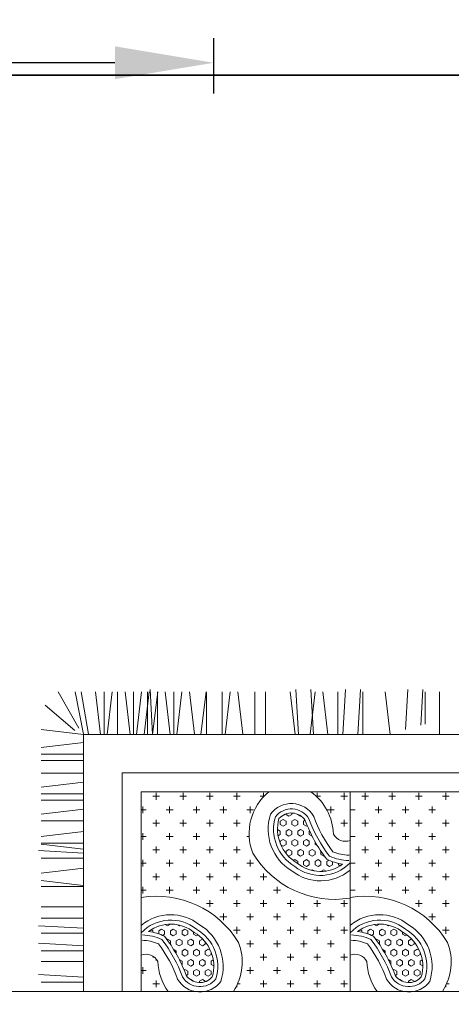
# Model space of a CAD drawing. Units: inches. Extents: x -638 to 186, y -762 to 59.
# Tile 18 of 31: x -135 to -118, y -243 to -203. Entities that reach past the tile are written whole.
import ezdxf

# ---------------------------------------------------------------- set-up
doc = ezdxf.new("R2010")
doc.units = ezdxf.units.IN
for name, color, linetype, lineweight in [('A-ANNO-DIMS', 2, 'Continuous', 18), ('furn', 8, 'Continuous', 13), ('wall', 7, 'Continuous', 35)]:
    doc.layers.add(name, color=color, linetype=linetype, lineweight=lineweight)
doc.styles.get("Standard").update_dxf_attribs({"font": 'arial.ttf'})
doc.dimstyles.new('ISO-25', dxfattribs={"dimtxt": 4, "dimasz": 4, "dimexe": 1.25, "dimexo": 0.625, "dimtad": 0, "dimlunit": 4, "dimtxsty": 'Standard', "dimcen": 2.5, "dimclrt": 256, "dimadec": 0, "dimazin": 0, "dimtfac": 1, "dimtmove": 0, "dimatfit": 3, "dimfxl": 1, "dimfxlon": 1, "dimarcsym": 0})

# ---------------------------------------------------------------- blocks, each defined once
blk = doc.blocks.new('BED-DOUBLE-WITH-NIGHTSTANDS')
for p, q in [((58.548, 11.244), (58.548, 59.951)), ((58.923, 31.914), (58.923, 33.642)), ((59.126, 31.914), (59.228, 33.743)), ((59.755, 31.928), (59.755, 33.639)), ((60.193, 31.914), (60.193, 33.642)), ((60.397, 31.914), (60.499, 33.743)), ((60.906, 31.914), (60.906, 33.642)), ((61.11, 31.914), (61.212, 33.743)), ((61.517, 31.914), (61.517, 33.642)), ((61.977, 31.914), (61.977, 33.642)), ((62.81, 31.928), (62.81, 33.639)), ((62.841, 31.928), (63.044, 33.642)), ((63.554, 31.914), (63.35, 33.642)), ((63.961, 31.914), (63.961, 33.642)), ((64.165, 31.914), (64.266, 33.743)), ((64.327, 31.928), (64.531, 33.642)), ((64.572, 31.914), (64.572, 33.642)), ((65.04, 31.914), (64.836, 33.642)), ((65.476, 31.914), (65.476, 33.642)), ((65.944, 31.914), (65.741, 33.642)), ((66.309, 31.928), (66.309, 33.639)), ((66.573, 31.914), (66.573, 33.642)), ((67.041, 31.914), (66.838, 33.642)), ((67.406, 31.928), (67.406, 33.639)), ((67.922, 31.928), (67.922, 33.639)), ((68.186, 31.914), (68.186, 33.642)), ((68.654, 31.914), (68.45, 33.642)), ((68.982, 31.914), (69.186, 33.642)), ((69.142, 32.273), (70.169, 33.468)), ((69.232, 32.112), (70.71, 32.951)), ((68.996, 31.914), (70.707, 32.257)), ((68.996, 31.721), (70.707, 32.011)), ((58.548, 31.914), (68.982, 31.914)), ((68.982, 31.914), (68.982, 1.829)), ((68.982, 31.232), (70.71, 31.436)), ((68.982, 30.966), (70.71, 30.762)), ((68.996, 31.086), (70.707, 31.086)), ((68.982, 30.547), (70.71, 30.547)), ((58.548, 30.359), (67.427, 30.359)), ((67.427, 30.359), (67.427, 3.384)), ((68.982, 30.033), (70.71, 30.237)), ((68.982, 29.767), (70.71, 29.563)), ((68.996, 29.887), (70.707, 29.887)), ((58.548, 29.582), (66.65, 29.582)), ((59.258, 29.515), (59.53, 29.515)), ((59.394, 29.379), (59.394, 29.582)), ((62.523, 29.515), (62.795, 29.515)), ((62.659, 29.379), (62.659, 29.582)), ((63.612, 29.515), (63.884, 29.515)), ((63.748, 29.379), (63.748, 29.582)), ((64.7, 29.515), (64.972, 29.515)), ((64.836, 29.379), (64.836, 29.582)), ((65.788, 29.515), (66.06, 29.515)), ((65.924, 29.379), (65.924, 29.582)), ((66.65, 29.582), (66.65, 4.161)), ((68.982, 29.46), (70.71, 29.256)), ((68.982, 29.324), (70.71, 29.324)), ((68.982, 29.121), (70.811, 29.223)), ((58.714, 28.971), (58.986, 28.971)), ((58.85, 28.835), (58.85, 29.107)), ((59.802, 28.971), (59.857, 28.971)), ((59.938, 29.054), (59.938, 29.107)), ((61.003, 28.869), (60.881, 28.869)), ((61.003, 29.104), (60.948, 29.104)), ((61.047, 29.18), (61.003, 29.104)), ((61.003, 28.869), (61.072, 28.751)), ((63.067, 28.971), (63.339, 28.971)), ((63.203, 28.835), (63.203, 29.107)), ((64.156, 28.971), (64.428, 28.971)), ((64.292, 28.835), (64.292, 29.107)), ((65.244, 28.971), (65.516, 28.971)), ((65.38, 28.835), (65.38, 29.107)), ((66.332, 28.971), (66.605, 28.971)), ((66.468, 28.835), (66.468, 29.107)), ((68.982, 28.917), (70.71, 28.917)), ((68.996, 29.116), (70.71, 28.912)), ((60.459, 28.399), (60.459, 28.397)), ((60.595, 28.397), (60.459, 28.397)), ((60.663, 28.515), (60.595, 28.397)), ((60.652, 28.534), (60.663, 28.515)), ((60.867, 28.397), (60.799, 28.28)), ((60.821, 28.713), (60.867, 28.633)), ((61.003, 28.633), (60.867, 28.633)), ((61.003, 28.397), (60.867, 28.397)), ((61.072, 28.751), (61.003, 28.633)), ((61.003, 28.397), (61.072, 28.28)), ((61.261, 28.608), (61.208, 28.515)), ((61.208, 28.515), (61.276, 28.397)), ((61.279, 28.397), (61.276, 28.397)), ((62.523, 28.427), (62.795, 28.427)), ((62.659, 28.291), (62.659, 28.563)), ((63.612, 28.427), (63.884, 28.427)), ((63.748, 28.291), (63.748, 28.563)), ((64.7, 28.427), (64.972, 28.427)), ((64.836, 28.291), (64.836, 28.563)), ((65.788, 28.427), (66.06, 28.427)), ((65.924, 28.291), (65.924, 28.563)), ((68.982, 28.403), (70.71, 28.606)), ((59.843, 28.037), (59.779, 27.926)), ((60.187, 28.162), (60.075, 28.162)), ((60.245, 28.262), (60.187, 28.162)), ((60.459, 28.162), (60.391, 28.044)), ((60.391, 28.044), (60.459, 27.926)), ((60.595, 28.162), (60.459, 28.162)), ((60.595, 28.162), (60.663, 28.044)), ((60.663, 28.044), (60.595, 27.926)), ((60.799, 28.28), (60.867, 28.162)), ((61.003, 28.162), (60.867, 28.162)), ((61.072, 28.28), (61.003, 28.162)), ((61.258, 28.131), (61.208, 28.044)), ((61.208, 28.044), (61.231, 28.004)), ((63.203, 27.747), (63.203, 28.019)), ((64.292, 27.747), (64.292, 28.019)), ((65.38, 27.747), (65.38, 28.019)), ((66.468, 27.747), (66.468, 28.019)), ((68.982, 28.136), (70.71, 27.933)), ((68.996, 28.256), (70.707, 28.256)), ((59.199, 27.753), (59.235, 27.69)), ((59.371, 27.69), (59.235, 27.69)), ((59.439, 27.808), (59.371, 27.69)), ((59.419, 27.842), (59.439, 27.808)), ((59.643, 27.69), (59.575, 27.573)), ((59.637, 27.937), (59.643, 27.926)), ((59.779, 27.926), (59.643, 27.926)), ((59.779, 27.69), (59.643, 27.69)), ((59.779, 27.69), (59.847, 27.573)), ((60.051, 27.926), (59.983, 27.808)), ((59.983, 27.808), (60.051, 27.69)), ((60.187, 27.926), (60.051, 27.926)), ((60.187, 27.69), (60.051, 27.69)), ((60.187, 27.926), (60.255, 27.808)), ((60.255, 27.808), (60.187, 27.69)), ((60.459, 27.69), (60.391, 27.573)), ((60.595, 27.926), (60.459, 27.926)), ((60.595, 27.69), (60.459, 27.69)), ((60.595, 27.69), (60.663, 27.573)), ((60.867, 27.926), (60.799, 27.808)), ((60.799, 27.808), (60.867, 27.69)), ((61.003, 27.926), (60.867, 27.926)), ((61.003, 27.69), (60.867, 27.69)), ((61.003, 27.926), (61.072, 27.808)), ((61.072, 27.808), (61.003, 27.69)), ((63.067, 27.883), (63.339, 27.883)), ((64.156, 27.883), (64.428, 27.883)), ((65.244, 27.883), (65.516, 27.883)), ((66.332, 27.883), (66.605, 27.883)), ((68.996, 27.424), (70.71, 27.627)), ((58.963, 27.219), (58.904, 27.219)), ((58.963, 27.455), (58.955, 27.455)), ((59.031, 27.573), (58.963, 27.455)), ((58.963, 27.219), (59.031, 27.101)), ((59.025, 27.583), (59.031, 27.573)), ((59.235, 27.455), (59.167, 27.337)), ((59.167, 27.337), (59.235, 27.219)), ((59.371, 27.455), (59.235, 27.455)), ((59.371, 27.219), (59.235, 27.219)), ((59.371, 27.455), (59.439, 27.337)), ((59.439, 27.337), (59.371, 27.219)), ((59.575, 27.573), (59.643, 27.455)), ((59.643, 27.219), (59.575, 27.101)), ((59.779, 27.455), (59.643, 27.455)), ((59.779, 27.219), (59.643, 27.219)), ((59.847, 27.573), (59.779, 27.455)), ((59.779, 27.219), (59.847, 27.101)), ((60.051, 27.455), (59.983, 27.337)), ((59.983, 27.337), (60.051, 27.219)), ((60.187, 27.455), (60.051, 27.455)), ((60.187, 27.219), (60.051, 27.219)), ((60.187, 27.455), (60.255, 27.337)), ((60.255, 27.337), (60.187, 27.219)), ((60.391, 27.573), (60.459, 27.455)), ((60.459, 27.219), (60.391, 27.101)), ((60.595, 27.455), (60.459, 27.455)), ((60.595, 27.219), (60.459, 27.219)), ((60.663, 27.573), (60.595, 27.455)), ((60.595, 27.219), (60.663, 27.101)), ((60.867, 27.455), (60.799, 27.337)), ((60.799, 27.337), (60.836, 27.274)), ((60.958, 27.455), (60.867, 27.455)), ((62.523, 27.339), (62.795, 27.339)), ((62.659, 27.203), (62.659, 27.475)), ((63.612, 27.339), (63.884, 27.339)), ((63.748, 27.203), (63.748, 27.475)), ((64.7, 27.339), (64.972, 27.339)), ((64.836, 27.203), (64.836, 27.475)), ((65.788, 27.339), (66.06, 27.339)), ((65.924, 27.203), (65.924, 27.475)), ((58.963, 26.984), (58.94, 26.984)), ((59.031, 27.101), (58.963, 26.984)), ((59.235, 26.984), (59.167, 26.866)), ((59.167, 26.866), (59.235, 26.748)), ((59.371, 26.984), (59.235, 26.984)), ((59.371, 26.984), (59.439, 26.866)), ((59.439, 26.866), (59.371, 26.748)), ((59.575, 27.101), (59.643, 26.984)), ((59.779, 26.984), (59.643, 26.984)), ((59.847, 27.101), (59.779, 26.984)), ((60.051, 26.984), (59.983, 26.866)), ((59.983, 26.866), (60.051, 26.748)), ((60.187, 26.984), (60.051, 26.984)), ((60.187, 26.984), (60.255, 26.866)), ((60.255, 26.866), (60.201, 26.772)), ((60.391, 27.101), (60.459, 26.984)), ((60.553, 26.984), (60.459, 26.984)), ((60.663, 27.101), (60.637, 27.055)), ((61.979, 26.795), (62.251, 26.795)), ((62.115, 26.659), (62.115, 26.931)), ((63.067, 26.795), (63.339, 26.795)), ((63.203, 26.659), (63.203, 26.931)), ((64.156, 26.795), (64.428, 26.795)), ((64.292, 26.659), (64.292, 26.931)), ((65.244, 26.795), (65.516, 26.795)), ((65.38, 26.659), (65.38, 26.931)), ((66.332, 26.795), (66.605, 26.795)), ((66.468, 26.659), (66.468, 26.931)), ((68.996, 27.156), (70.71, 26.953)), ((68.996, 26.933), (70.707, 26.933)), ((59.371, 26.748), (59.235, 26.748)), ((59.643, 26.748), (59.58, 26.638)), ((59.779, 26.748), (59.643, 26.748)), ((59.779, 26.748), (59.83, 26.661)), ((60.144, 26.748), (60.051, 26.748)), ((61.435, 26.25), (61.707, 26.25)), ((61.571, 26.114), (61.571, 26.386)), ((62.523, 26.25), (62.795, 26.25)), ((62.659, 26.114), (62.659, 26.386)), ((63.612, 26.25), (63.884, 26.25)), ((63.748, 26.114), (63.748, 26.386)), ((64.7, 26.25), (64.972, 26.25)), ((64.836, 26.114), (64.836, 26.386)), ((65.788, 26.25), (66.06, 26.25)), ((65.924, 26.114), (65.924, 26.386)), ((68.982, 26.177), (70.71, 25.974)), ((68.996, 26.297), (70.707, 26.297)), ((58.714, 25.706), (58.783, 25.706)), ((58.85, 25.57), (58.85, 25.675)), ((60.891, 25.706), (61.163, 25.706)), ((61.027, 25.57), (61.027, 25.842)), ((61.979, 25.706), (62.251, 25.706)), ((62.115, 25.57), (62.115, 25.842)), ((63.067, 25.706), (63.339, 25.706)), ((63.203, 25.57), (63.203, 25.842)), ((64.156, 25.706), (64.428, 25.706)), ((64.292, 25.57), (64.292, 25.842)), ((65.244, 25.706), (65.516, 25.706)), ((65.38, 25.57), (65.38, 25.842)), ((66.332, 25.706), (66.605, 25.706)), ((66.468, 25.57), (66.468, 25.842)), ((68.996, 25.465), (70.71, 25.668)), ((59.394, 25.026), (59.394, 25.298)), ((60.483, 25.026), (60.483, 25.298)), ((61.571, 25.026), (61.571, 25.298)), ((62.659, 25.026), (62.659, 25.298)), ((63.748, 25.026), (63.748, 25.298)), ((64.836, 25.2), (64.836, 25.298)), ((65.924, 25.026), (65.924, 25.298)), ((59.258, 25.162), (59.53, 25.162)), ((60.346, 25.162), (60.619, 25.162)), ((61.435, 25.162), (61.707, 25.162)), ((62.523, 25.162), (62.795, 25.162)), ((63.612, 25.162), (63.884, 25.162)), ((65.788, 25.162), (66.06, 25.162)), ((68.996, 24.973), (70.707, 24.973)), ((58.714, 24.618), (58.986, 24.618)), ((58.85, 24.482), (58.85, 24.754)), ((59.802, 24.618), (60.074, 24.618)), ((59.938, 24.482), (59.938, 24.754)), ((60.891, 24.618), (61.163, 24.618)), ((61.027, 24.482), (61.027, 24.754)), ((61.979, 24.618), (62.251, 24.618)), ((62.115, 24.482), (62.115, 24.754)), ((63.067, 24.618), (63.339, 24.618)), ((63.203, 24.482), (63.203, 24.754)), ((66.45, 24.618), (66.605, 24.618)), ((66.468, 24.601), (66.468, 24.754)), ((68.996, 24.543), (70.707, 24.543)), ((59.258, 24.074), (59.53, 24.074)), ((59.394, 23.938), (59.394, 24.21)), ((60.346, 24.074), (60.619, 24.074)), ((60.483, 23.938), (60.483, 24.21)), ((61.435, 24.074), (61.707, 24.074)), ((61.571, 23.938), (61.571, 24.21)), ((62.523, 24.074), (62.795, 24.074)), ((62.659, 23.938), (62.659, 24.21)), ((64.917, 23.942), (64.866, 24.03)), ((65.053, 23.942), (65.116, 24.052)), ((58.85, 23.393), (58.85, 23.666)), ((59.938, 23.393), (59.938, 23.666)), ((61.027, 23.393), (61.027, 23.666)), ((62.115, 23.393), (62.115, 23.666)), ((64.032, 23.589), (64.059, 23.635)), ((64.143, 23.707), (64.236, 23.707)), ((64.304, 23.589), (64.236, 23.707)), ((64.44, 23.825), (64.495, 23.919)), ((64.508, 23.707), (64.44, 23.825)), ((64.508, 23.707), (64.644, 23.707)), ((64.552, 23.942), (64.644, 23.942)), ((64.712, 23.825), (64.644, 23.942)), ((64.644, 23.707), (64.712, 23.825)), ((64.849, 23.589), (64.917, 23.707)), ((64.917, 23.942), (65.053, 23.942)), ((64.917, 23.707), (65.053, 23.707)), ((65.121, 23.589), (65.053, 23.707)), ((65.257, 23.825), (65.325, 23.942)), ((65.325, 23.707), (65.257, 23.825)), ((65.325, 23.942), (65.461, 23.942)), ((65.325, 23.707), (65.461, 23.707)), ((65.529, 23.825), (65.461, 23.942)), ((65.461, 23.707), (65.529, 23.825)), ((65.665, 23.589), (65.733, 23.707)), ((65.733, 23.707), (65.755, 23.707)), ((58.714, 23.53), (58.986, 23.53)), ((59.802, 23.53), (60.074, 23.53)), ((60.891, 23.53), (61.163, 23.53)), ((61.979, 23.53), (62.251, 23.53)), ((63.737, 23.235), (63.828, 23.235)), ((63.828, 23.235), (63.896, 23.353)), ((63.896, 23.353), (63.86, 23.416)), ((64.1, 23.471), (64.032, 23.589)), ((64.032, 23.118), (64.1, 23.235)), ((64.1, 23.471), (64.236, 23.471)), ((64.1, 23.235), (64.236, 23.235)), ((64.236, 23.471), (64.304, 23.589)), ((64.304, 23.118), (64.236, 23.235)), ((64.44, 23.353), (64.508, 23.471)), ((64.508, 23.235), (64.44, 23.353)), ((64.508, 23.471), (64.644, 23.471)), ((64.508, 23.235), (64.644, 23.235)), ((64.712, 23.353), (64.644, 23.471)), ((64.644, 23.235), (64.712, 23.353)), ((64.917, 23.471), (64.849, 23.589)), ((64.849, 23.118), (64.917, 23.235)), ((64.917, 23.471), (65.053, 23.471)), ((64.917, 23.235), (65.053, 23.235)), ((65.053, 23.471), (65.121, 23.589)), ((65.121, 23.118), (65.053, 23.235)), ((65.257, 23.353), (65.325, 23.471)), ((65.325, 23.235), (65.257, 23.353)), ((65.325, 23.471), (65.461, 23.471)), ((65.325, 23.235), (65.461, 23.235)), ((65.529, 23.353), (65.461, 23.471)), ((65.461, 23.235), (65.529, 23.353)), ((65.733, 23.471), (65.665, 23.589)), ((65.665, 23.118), (65.733, 23.235)), ((65.733, 23.471), (65.791, 23.471)), ((65.733, 23.235), (65.741, 23.235)), ((68.982, 23.339), (70.71, 23.542)), ((68.982, 23.207), (70.811, 23.309)), ((59.258, 22.985), (59.53, 22.985)), ((59.394, 22.849), (59.394, 23.121)), ((60.346, 22.985), (60.619, 22.985)), ((60.483, 22.849), (60.483, 23.121)), ((61.435, 22.985), (61.707, 22.985)), ((61.571, 22.849), (61.571, 23.121)), ((63.624, 22.882), (63.692, 23)), ((63.692, 22.764), (63.624, 22.882)), ((63.692, 23), (63.828, 23)), ((63.896, 22.882), (63.828, 23)), ((63.828, 22.764), (63.896, 22.882)), ((64.1, 23), (64.032, 23.118)), ((64.1, 23), (64.236, 23)), ((64.236, 23), (64.304, 23.118)), ((64.44, 22.882), (64.508, 23)), ((64.508, 22.764), (64.44, 22.882)), ((64.508, 23), (64.644, 23)), ((64.712, 22.882), (64.644, 23)), ((64.644, 22.764), (64.712, 22.882)), ((64.917, 23), (64.849, 23.118)), ((64.917, 23), (65.053, 23)), ((65.053, 23), (65.121, 23.118)), ((65.257, 22.882), (65.325, 23)), ((65.276, 22.848), (65.257, 22.882)), ((65.325, 23), (65.461, 23)), ((65.497, 22.937), (65.461, 23)), ((65.671, 23.107), (65.665, 23.118)), ((58.714, 22.441), (58.986, 22.441)), ((58.85, 22.305), (58.85, 22.577)), ((59.802, 22.441), (60.074, 22.441)), ((59.938, 22.305), (59.938, 22.577)), ((60.891, 22.441), (61.163, 22.441)), ((61.027, 22.305), (61.027, 22.577)), ((61.979, 22.441), (62.251, 22.441)), ((62.115, 22.305), (62.115, 22.577)), ((63.438, 22.559), (63.488, 22.646)), ((63.488, 22.646), (63.465, 22.686)), ((63.624, 22.411), (63.692, 22.529)), ((63.692, 22.293), (63.624, 22.411)), ((63.692, 22.764), (63.828, 22.764)), ((63.692, 22.529), (63.828, 22.529)), ((63.896, 22.411), (63.828, 22.529)), ((63.828, 22.293), (63.896, 22.411)), ((64.032, 22.646), (64.1, 22.764)), ((64.1, 22.529), (64.032, 22.646)), ((64.1, 22.764), (64.236, 22.764)), ((64.1, 22.529), (64.236, 22.529)), ((64.304, 22.646), (64.236, 22.764)), ((64.236, 22.529), (64.304, 22.646)), ((64.451, 22.428), (64.508, 22.529)), ((64.508, 22.764), (64.644, 22.764)), ((64.508, 22.529), (64.621, 22.529)), ((64.852, 22.653), (64.917, 22.764)), ((64.917, 22.764), (65.053, 22.764)), ((65.059, 22.753), (65.053, 22.764)), ((66.43, 22.441), (66.605, 22.441)), ((66.468, 22.305), (66.468, 22.481)), ((68.982, 22.596), (70.811, 22.698)), ((68.996, 22.728), (70.71, 22.524)), ((59.394, 21.761), (59.394, 22.033)), ((60.483, 21.761), (60.483, 22.033)), ((61.571, 21.761), (61.571, 22.033)), ((63.417, 22.293), (63.42, 22.293)), ((63.488, 22.175), (63.42, 22.293)), ((63.434, 22.082), (63.488, 22.175)), ((63.624, 21.939), (63.692, 22.057)), ((63.692, 22.293), (63.828, 22.293)), ((63.692, 22.057), (63.828, 22.057)), ((63.874, 21.977), (63.828, 22.057)), ((64.032, 22.175), (64.1, 22.293)), ((64.043, 22.156), (64.032, 22.175)), ((64.1, 22.293), (64.236, 22.293)), ((64.237, 22.292), (64.236, 22.293)), ((65.924, 21.761), (65.924, 22.033)), ((68.982, 22.015), (70.71, 22.219)), ((59.258, 21.897), (59.53, 21.897)), ((60.346, 21.897), (60.619, 21.897)), ((61.435, 21.897), (61.707, 21.897)), ((63.692, 21.822), (63.624, 21.939)), ((63.692, 21.822), (63.815, 21.822)), ((65.788, 21.897), (66.06, 21.897)), ((68.982, 21.608), (70.71, 21.608)), ((58.714, 21.353), (58.986, 21.353)), ((58.85, 21.217), (58.85, 21.489)), ((59.802, 21.353), (60.074, 21.353)), ((59.938, 21.217), (59.938, 21.489)), ((60.891, 21.353), (61.163, 21.353)), ((61.027, 21.217), (61.027, 21.489)), ((61.979, 21.353), (62.251, 21.353)), ((62.115, 21.217), (62.115, 21.489)), ((63.648, 21.51), (63.692, 21.586)), ((63.692, 21.586), (63.748, 21.586)), ((65.244, 21.353), (65.516, 21.353)), ((65.38, 21.217), (65.38, 21.489)), ((66.332, 21.353), (66.605, 21.353)), ((66.468, 21.217), (66.468, 21.489)), ((68.982, 21.404), (70.811, 21.302)), ((58.548, 21.108), (66.65, 21.108)), ((62.659, 20.906), (62.659, 21.108)), ((63.748, 20.906), (63.748, 21.108)), ((64.836, 20.906), (64.836, 21.108)), ((65.924, 20.906), (65.924, 21.108)), ((68.982, 20.793), (70.811, 20.691)), ((61.003, 20.395), (60.881, 20.395)), ((61.003, 20.631), (60.948, 20.631)), ((61.047, 20.707), (61.003, 20.631)), ((61.003, 20.395), (61.072, 20.277)), ((63.067, 20.498), (63.339, 20.498)), ((63.203, 20.362), (63.203, 20.634)), ((64.156, 20.498), (64.428, 20.498)), ((64.292, 20.362), (64.292, 20.634)), ((65.244, 20.498), (65.516, 20.498)), ((65.38, 20.362), (65.38, 20.634)), ((66.332, 20.498), (66.605, 20.498)), ((66.468, 20.362), (66.468, 20.634)), ((68.982, 20.59), (70.71, 20.59)), ((60.663, 20.042), (60.595, 19.924)), ((60.652, 20.061), (60.663, 20.042)), ((60.821, 20.239), (60.867, 20.159)), ((61.003, 20.159), (60.867, 20.159)), ((61.072, 20.277), (61.003, 20.159)), ((61.261, 20.135), (61.208, 20.042)), ((61.208, 20.042), (61.276, 19.924)), ((62.659, 19.817), (62.659, 20.09)), ((63.748, 19.817), (63.748, 20.09)), ((64.836, 19.817), (64.836, 20.09)), ((65.924, 19.817), (65.924, 20.09)), ((60.187, 19.688), (60.075, 19.688)), ((60.245, 19.788), (60.187, 19.688)), ((60.459, 19.688), (60.391, 19.57)), ((60.459, 19.925), (60.459, 19.924)), ((60.595, 19.924), (60.459, 19.924)), ((60.595, 19.688), (60.459, 19.688)), ((60.595, 19.688), (60.663, 19.57)), ((60.867, 19.924), (60.799, 19.806)), ((60.799, 19.806), (60.867, 19.688)), ((61.003, 19.924), (60.867, 19.924)), ((61.003, 19.688), (60.867, 19.688)), ((61.003, 19.924), (61.072, 19.806)), ((61.072, 19.806), (61.003, 19.688)), ((61.258, 19.657), (61.208, 19.57)), ((61.279, 19.924), (61.276, 19.924)), ((62.523, 19.954), (62.795, 19.954)), ((63.612, 19.954), (63.884, 19.954)), ((64.7, 19.954), (64.972, 19.954)), ((65.788, 19.954), (66.06, 19.954)), ((68.982, 19.485), (70.71, 19.689)), ((59.199, 19.28), (59.235, 19.217)), ((59.371, 19.217), (59.235, 19.217)), ((59.439, 19.335), (59.371, 19.217)), ((59.419, 19.369), (59.439, 19.335)), ((59.643, 19.217), (59.575, 19.099)), ((59.637, 19.464), (59.643, 19.453)), ((59.779, 19.453), (59.643, 19.453)), ((59.779, 19.217), (59.643, 19.217)), ((59.843, 19.564), (59.779, 19.453)), ((59.779, 19.217), (59.847, 19.099)), ((60.051, 19.453), (59.983, 19.335)), ((59.983, 19.335), (60.051, 19.217)), ((60.187, 19.453), (60.051, 19.453)), ((60.187, 19.217), (60.051, 19.217)), ((60.187, 19.453), (60.255, 19.335)), ((60.255, 19.335), (60.187, 19.217)), ((60.391, 19.57), (60.459, 19.453)), ((60.459, 19.217), (60.391, 19.099)), ((60.595, 19.453), (60.459, 19.453)), ((60.595, 19.217), (60.459, 19.217)), ((60.663, 19.57), (60.595, 19.453)), ((60.595, 19.217), (60.663, 19.099)), ((60.867, 19.453), (60.799, 19.335)), ((60.799, 19.335), (60.867, 19.217)), ((61.003, 19.453), (60.867, 19.453)), ((61.003, 19.217), (60.867, 19.217)), ((61.003, 19.453), (61.072, 19.335)), ((61.072, 19.335), (61.003, 19.217)), ((61.208, 19.57), (61.231, 19.53)), ((63.067, 19.409), (63.339, 19.409)), ((63.203, 19.273), (63.203, 19.545)), ((64.156, 19.409), (64.428, 19.409)), ((64.292, 19.273), (64.292, 19.545)), ((65.244, 19.409), (65.516, 19.409)), ((65.38, 19.273), (65.38, 19.545)), ((66.332, 19.409), (66.605, 19.409)), ((66.468, 19.273), (66.468, 19.545)), ((58.963, 18.981), (58.955, 18.981)), ((59.031, 19.099), (58.963, 18.981)), ((59.025, 19.109), (59.031, 19.099)), ((59.235, 18.981), (59.167, 18.863)), ((59.167, 18.863), (59.235, 18.746)), ((59.371, 18.981), (59.235, 18.981)), ((59.371, 18.981), (59.439, 18.863)), ((59.439, 18.863), (59.371, 18.746)), ((59.575, 19.099), (59.643, 18.981)), ((59.779, 18.981), (59.643, 18.981)), ((59.847, 19.099), (59.779, 18.981)), ((60.051, 18.981), (59.983, 18.863)), ((59.983, 18.863), (60.051, 18.746)), ((60.187, 18.981), (60.051, 18.981)), ((60.187, 18.981), (60.255, 18.863)), ((60.255, 18.863), (60.187, 18.746)), ((60.391, 19.099), (60.459, 18.981)), ((60.595, 18.981), (60.459, 18.981)), ((60.663, 19.099), (60.595, 18.981)), ((60.867, 18.981), (60.799, 18.863)), ((60.799, 18.863), (60.836, 18.801)), ((60.958, 18.981), (60.867, 18.981)), ((62.523, 18.865), (62.795, 18.865)), ((62.659, 18.729), (62.659, 19.001)), ((63.612, 18.865), (63.884, 18.865)), ((63.748, 18.729), (63.748, 19.001)), ((64.7, 18.865), (64.972, 18.865)), ((64.836, 18.729), (64.836, 19.001)), ((65.788, 18.865), (66.06, 18.865)), ((65.924, 18.729), (65.924, 19.001)), ((69.184, 18.863), (70.811, 18.772)), ((58.963, 18.746), (58.904, 18.746)), ((58.963, 18.51), (58.94, 18.51)), ((58.963, 18.746), (59.031, 18.628)), ((59.031, 18.628), (58.963, 18.51)), ((59.235, 18.51), (59.167, 18.392)), ((59.167, 18.392), (59.235, 18.274)), ((59.371, 18.746), (59.235, 18.746)), ((59.371, 18.51), (59.235, 18.51)), ((59.371, 18.51), (59.439, 18.392)), ((59.439, 18.392), (59.371, 18.274)), ((59.643, 18.746), (59.575, 18.628)), ((59.575, 18.628), (59.643, 18.51)), ((59.779, 18.746), (59.643, 18.746)), ((59.779, 18.51), (59.643, 18.51)), ((59.779, 18.746), (59.847, 18.628)), ((59.847, 18.628), (59.779, 18.51)), ((60.051, 18.51), (59.983, 18.392)), ((59.983, 18.392), (60.051, 18.274)), ((60.187, 18.746), (60.051, 18.746)), ((60.187, 18.51), (60.051, 18.51)), ((60.187, 18.51), (60.255, 18.392)), ((60.255, 18.392), (60.201, 18.298)), ((60.459, 18.746), (60.391, 18.628)), ((60.391, 18.628), (60.459, 18.51)), ((60.595, 18.746), (60.459, 18.746)), ((60.553, 18.51), (60.459, 18.51)), ((60.595, 18.746), (60.663, 18.628)), ((60.663, 18.628), (60.637, 18.582)), ((62.115, 18.185), (62.115, 18.457)), ((63.203, 18.185), (63.203, 18.457)), ((64.292, 18.185), (64.292, 18.457)), ((65.38, 18.185), (65.38, 18.457)), ((66.468, 18.185), (66.468, 18.457)), ((59.371, 18.274), (59.235, 18.274)), ((59.643, 18.274), (59.58, 18.165)), ((59.779, 18.274), (59.643, 18.274)), ((59.779, 18.274), (59.83, 18.187)), ((60.144, 18.274), (60.051, 18.274)), ((61.979, 18.321), (62.251, 18.321)), ((63.067, 18.321), (63.339, 18.321)), ((64.156, 18.321), (64.428, 18.321)), ((65.244, 18.321), (65.516, 18.321)), ((66.332, 18.321), (66.605, 18.321)), ((69.357, 18.243), (70.811, 18.162)), ((69.393, 18.06), (70.71, 18.06)), ((61.435, 17.777), (61.707, 17.777)), ((61.571, 17.641), (61.571, 17.913)), ((62.523, 17.777), (62.795, 17.777)), ((62.659, 17.641), (62.659, 17.913)), ((63.612, 17.777), (63.884, 17.777)), ((63.748, 17.641), (63.748, 17.913)), ((64.7, 17.777), (64.972, 17.777)), ((64.836, 17.641), (64.836, 17.913)), ((65.788, 17.777), (66.06, 17.777)), ((65.924, 17.641), (65.924, 17.913)), ((58.714, 17.233), (58.783, 17.233)), ((58.85, 17.097), (58.85, 17.202)), ((60.891, 17.233), (61.163, 17.233)), ((61.027, 17.097), (61.027, 17.369)), ((61.979, 17.233), (62.251, 17.233)), ((62.115, 17.097), (62.115, 17.369)), ((63.067, 17.233), (63.339, 17.233)), ((63.203, 17.097), (63.203, 17.369)), ((64.156, 17.233), (64.428, 17.233)), ((64.292, 17.097), (64.292, 17.369)), ((65.244, 17.233), (65.516, 17.233)), ((65.38, 17.097), (65.38, 17.369)), ((66.332, 17.233), (66.605, 17.233)), ((66.468, 17.097), (66.468, 17.369)), ((68.982, 17.492), (70.707, 17.492))]:
    blk.add_line(p, q)
for centre, radius, start, end in [((59.514, 29.388), 0.54, 297.0088, 21.0409), ((58.736, 29.604), 1.887, 337.4091, 358.0373), ((58.53, 28.957), 3.88, 301.1125, 9.2666), ((58.736, 29.604), 2.104, 335.7609, 358.0373), ((58.736, 29.604), 2.268, 334.7059, 351.7535), ((59.782, 28.381), 1.66, 321.1107, 46.3387), ((59.782, 28.381), 1.497, 320.6541, 36.833), ((59.782, 28.381), 1.878, 321.5973, 39.7611), ((59.856, 26.664), 2.246, 92.4675, 125.6302), ((57.143, 33.342), 5.571, 289.9219, 306.7677), ((57.143, 33.342), 5.789, 290.1318, 307.346), ((57.143, 33.342), 5.952, 290.2997, 307.7385), ((59.57, 27.2), 1.047, 120.344, 234.0192), ((59.57, 27.2), 0.829, 121.6232, 231.6957), ((59.57, 27.2), 0.666, 122.9498, 229.099), ((59.563, 28.229), 1.972, 252.055, 329.019), ((59.563, 28.229), 1.754, 253.2189, 329.4808), ((59.563, 28.229), 1.591, 254.3738, 329.9117), ((59.74, 27.689), 2.202, 237.1993, 291.1583), ((64.955, 23.002), 2.202, 39.6653, 111.1583), ((66.165, 21.733), 3.88, 121.1125, 189.2666), ((65.133, 22.461), 1.972, 72.055, 149.019), ((65.133, 22.461), 1.754, 73.2189, 149.4808), ((65.133, 22.461), 1.591, 74.3738, 149.9117), ((65.126, 23.49), 0.666, 302.9498, 49.099), ((65.126, 23.49), 0.829, 301.6232, 51.6957), ((65.126, 23.49), 1.047, 300.344, 54.0192), ((64.914, 22.31), 1.878, 141.5973, 219.7611), ((64.914, 22.31), 1.66, 141.1107, 226.3387), ((64.914, 22.31), 1.497, 140.6541, 216.833), ((67.553, 17.348), 5.952, 110.2997, 127.7385), ((67.553, 17.348), 5.789, 110.1318, 127.346), ((67.553, 17.348), 5.571, 109.9219, 126.7677), ((64.84, 24.027), 2.246, 272.4675, 323.7193), ((65.96, 21.087), 2.268, 154.7059, 171.7535), ((65.96, 21.087), 2.104, 155.7609, 178.0373), ((65.96, 21.087), 1.887, 157.4091, 178.0373), ((65.181, 21.302), 0.54, 117.0088, 201.0409), ((59.514, 20.915), 0.54, 297.0088, 21.0409), ((58.736, 21.13), 1.887, 337.4091, 358.0373), ((58.53, 20.484), 3.88, 301.1125, 9.2666), ((58.736, 21.13), 2.104, 335.7609, 358.0373), ((58.736, 21.13), 2.268, 334.7059, 351.7535), ((59.782, 19.907), 1.66, 321.1107, 46.3387), ((59.782, 19.907), 1.497, 320.6541, 36.833), ((59.782, 19.907), 1.878, 321.5973, 39.7611), ((59.856, 18.19), 2.246, 92.4675, 125.6302), ((57.143, 24.868), 5.571, 289.9219, 306.7677), ((57.143, 24.868), 5.789, 290.1318, 307.346), ((57.143, 24.868), 5.952, 290.2997, 307.7385), ((59.57, 18.727), 1.047, 120.344, 234.0192), ((59.57, 18.727), 0.829, 121.6232, 231.6957), ((59.57, 18.727), 0.666, 122.9498, 229.099), ((59.563, 19.756), 1.754, 253.2189, 329.4808), ((59.563, 19.756), 1.591, 254.3738, 329.9117), ((59.563, 19.756), 1.972, 252.055, 329.019), ((59.74, 19.215), 2.202, 237.1993, 291.1583)]:
    blk.add_arc(centre, radius, start, end)
blk = doc.blocks.new('*D23')
at = {"layer": 'A-ANNO-DIMS', "color": 0, "lineweight": -2, "transparency": 16777216}
for p, q in [((-165.015, -204.032), (-165.015, -206.282)), ((-127.219, -204.032), (-127.219, -206.282)), ((-165.015, -205.032), (-169.015, -205.032)), ((-131.219, -205.032), (-161.015, -205.032))]:
    blk.add_line(p, q, dxfattribs=at)
at = {"layer": 'A-ANNO-DIMS', "color": 0, "lineweight": 30, "transparency": 16777216}
for points in [[(-161.015, -204.365), (-161.015, -205.699), (-165.015, -205.032)], [(-131.219, -204.365), (-131.219, -205.699), (-127.219, -205.032)]]:
    blk.add_solid(points, dxfattribs=at)
at = {"layer": 'Defpoints', "color": 0, "lineweight": 30, "transparency": 16777216}
for p in [(-165.015, -199.363), (-127.219, -199.363), (-165.015, -205.032)]:
    blk.add_point(p, dxfattribs=at)
at = {"layer": 'A-ANNO-DIMS', "transparency": 16777216, "insert": (-201.224, -205.032), "char_height": 4, "attachment_point": 5}
blk.add_mtext('SWING DOOR 3\'-2" TYP.', dxfattribs=at)
blk = doc.blocks.new('*D37')
at = {"layer": 'A-ANNO-DIMS', "color": 0, "lineweight": -2, "transparency": 16777216}
for p, q in [((182.663, -232.533), (184.913, -232.533)), ((183.663, -236.533), (183.663, -250.511)), ((183.663, -276.533), (183.663, -262.555)), ((182.663, -280.533), (184.913, -280.533))]:
    blk.add_line(p, q, dxfattribs=at)
at = {"layer": 'A-ANNO-DIMS', "color": 0, "lineweight": 30, "transparency": 16777216}
for points in [[(182.997, -236.533), (184.33, -236.533), (183.663, -232.533)], [(182.997, -276.533), (184.33, -276.533), (183.663, -280.533)]]:
    blk.add_solid(points, dxfattribs=at)
at = {"layer": 'Defpoints', "color": 0, "lineweight": 30, "transparency": 16777216}
for p in [(-404.526, -232.533), (-404.526, -280.533), (183.663, -280.533)]:
    blk.add_point(p, dxfattribs=at)
at = {"layer": 'A-ANNO-DIMS', "transparency": 16777216, "insert": (183.663, -256.533), "char_height": 4, "attachment_point": 5, "rotation": 90}
blk.add_mtext('4\'-0"', dxfattribs=at)
blk = doc.blocks.new('*D56')
at = {"layer": 'A-ANNO-DIMS', "color": 0, "lineweight": -2, "transparency": 16777216}
for p, q in [((-165.026, 52.017), (-165.026, 54.267)), ((-100.526, 52.017), (-100.526, 54.267)), ((-161.026, 53.017), (-143.378, 53.017)), ((-104.526, 53.017), (-122.174, 53.017))]:
    blk.add_line(p, q, dxfattribs=at)
at = {"layer": 'A-ANNO-DIMS', "color": 0, "lineweight": 30, "transparency": 16777216}
for points in [[(-161.026, 53.684), (-161.026, 52.35), (-165.026, 53.017)], [(-104.526, 53.684), (-104.526, 52.35), (-100.526, 53.017)]]:
    blk.add_solid(points, dxfattribs=at)
at = {"layer": 'Defpoints', "color": 0, "lineweight": 30, "transparency": 16777216}
for p in [(-100.526, 53.017), (-165.026, -408.033), (-100.526, -408.033)]:
    blk.add_point(p, dxfattribs=at)
at = {"layer": 'A-ANNO-DIMS', "transparency": 16777216, "insert": (-132.776, 53.017), "char_height": 4, "attachment_point": 5}
blk.add_mtext('5\'-4 1/2"', dxfattribs=at)

msp = doc.modelspace()

# ---------------------------------------------------------------- linework, layer by layer
at = {"layer": 'wall'}
msp.add_line((-160.526, -205.533), (1.474, -205.533), dxfattribs=at)

# ---------------------------------------------------------------- block references
at = {"layer": 'furn', "rotation": 90.00000000000006}
msp.add_blockref('BED-DOUBLE-WITH-NIGHTSTANDS', (-100.575, -301.287), dxfattribs=at)

# ---------------------------------------------------------------- dimensions: what is measured, and where the dimension line sits
at = {"layer": 'A-ANNO-DIMS'}
dim = msp.add_linear_dim(base=(-100.526, 53.017), p1=(-165.026, -408.033), p2=(-100.526, -408.033), dimstyle='ISO-25', override={"dimdec": 1, "dimlfac": 1, "dimrnd": 0, "dimzin": 1, "dimdsep": 46, "dimlunit": 4, "dimfrac": 2}, dxfattribs=at)
dim.commit()
dim.dimension.update_dxf_attribs({"geometry": '*D56', "text_midpoint": (-132.776, 53.017)})
dim = msp.add_linear_dim(base=(-165.015, -205.032), p1=(-127.219, -199.363), p2=(-165.015, -199.363), angle=180, text='SWING DOOR <> TYP.', dimstyle='ISO-25', override={"dimdec": 1, "dimlfac": 1, "dimrnd": 0, "dimzin": 1, "dimdsep": 46, "dimlunit": 4, "dimfrac": 2}, dxfattribs=at)
dim.commit()
dim.dimension.update_dxf_attribs({"geometry": '*D23', "text_midpoint": (-201.224, -205.032)})
dim = msp.add_linear_dim(base=(183.663, -280.533), p1=(-404.526, -232.533), p2=(-404.526, -280.533), angle=90, dimstyle='ISO-25', override={"dimdec": 1, "dimlfac": 1, "dimrnd": 0, "dimzin": 1, "dimdsep": 46, "dimlunit": 4, "dimfrac": 2}, dxfattribs=at)
dim.commit()
dim.dimension.update_dxf_attribs({"geometry": '*D37', "text_midpoint": (183.663, -256.533)})

doc.saveas('drawing.dxf')
